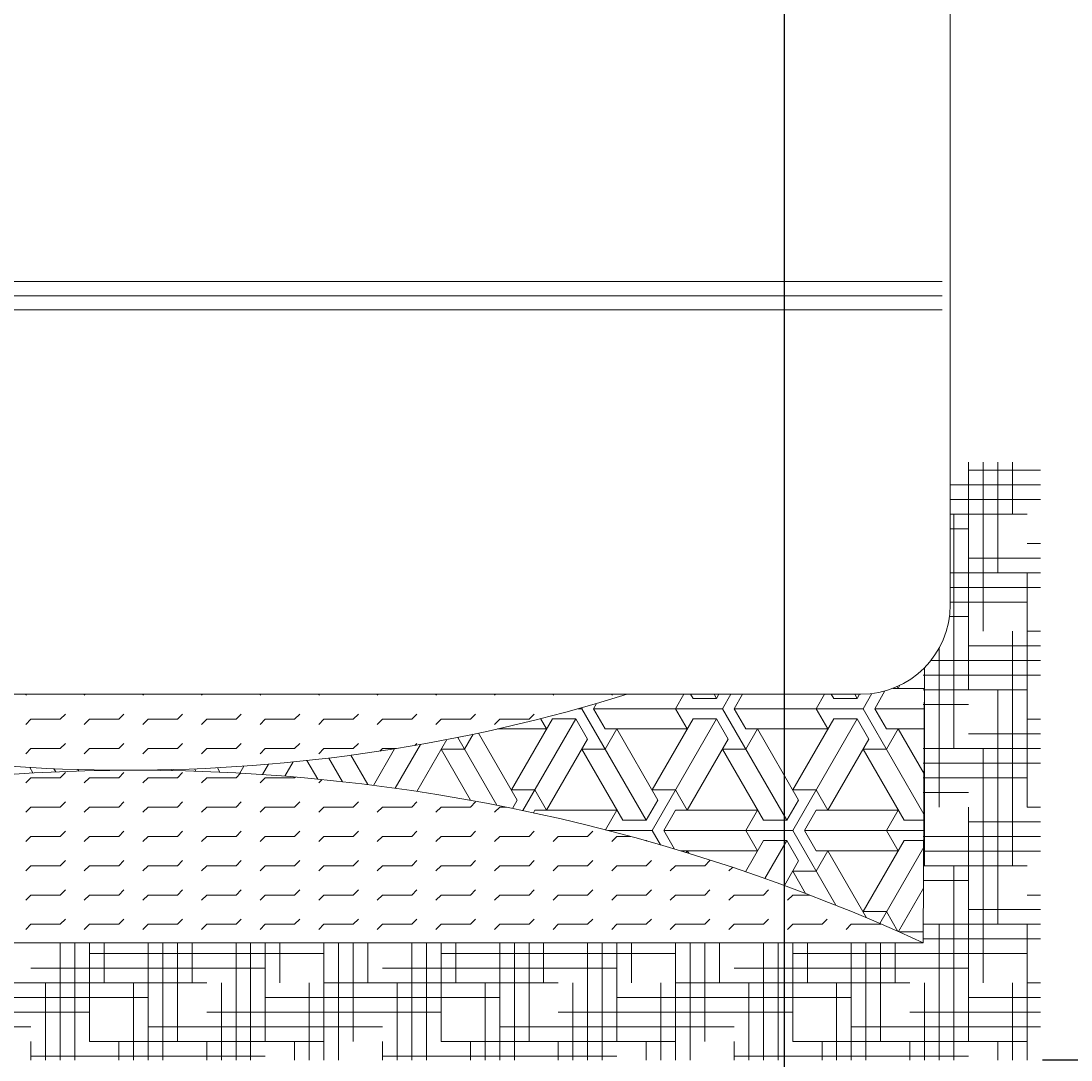
# Model space of a CAD drawing. Units: inches. Extents: x -1517 to -668, y -425 to 52.
# Tile 9 of 13: x -1161 to -1129, y -63 to -32. Entities that reach past the tile are written whole.
import ezdxf

# ---------------------------------------------------------------- set-up
doc = ezdxf.new("R2010")
doc.units = ezdxf.units.IN
doc.header["$MEASUREMENT"] = 0
doc.layers.add('A-ANNO-DIMS', color=2, linetype='Continuous', lineweight=18)
doc.layers.add('furniture block', color=8, linetype='Continuous', lineweight=18)
doc.styles.get("Standard").update_dxf_attribs({"font": 'arial.ttf'})
doc.dimstyles.get("Standard").update_dxf_attribs({"dimtxt": 0.18, "dimasz": 0.18, "dimexe": 0.18, "dimexo": 0.0625, "dimgap": 0.09, "dimtad": 0, "dimtih": 1, "dimtoh": 1, "dimdec": 4, "dimzin": 0, "dimdsep": 46, "dimlunit": 4, "dimtxsty": 'Standard', "dimcen": 0.09, "dimadec": 0, "dimazin": 0, "dimtfac": 1, "dimtdec": 4, "dimtofl": 0, "dimtmove": 0, "dimatfit": 3, "dimfxl": 1, "dimtolj": 1, "dimtzin": 0, "dimarcsym": 0})

# ---------------------------------------------------------------- blocks, each defined once
blk = doc.blocks.new('A$C62731D1C')
for p, q in [((1.46787, 2.14084, 0.68571), (1.46787, 0.38824, 0.68571)), ((0.10613, 0.66415, 0.68571), (1.46095, 0.66415, 0.68571)), ((0.10613, 0.65215, 0.68571), (1.46095, 0.65215, 0.68571)), ((0.10613, 0.64015, 0.68571), (1.46095, 0.64015, 0.68571)), ((1.4835, 0.31577, 0.68571), (1.4835, 0.50998, 0.68571)), ((1.4835, 0.50327, 0.68571), (1.54488, 0.50327, 0.68571)), ((1.496, 0.36577, 0.68571), (1.496, 0.50998, 0.68571)), ((1.5085, 0.41577, 0.68571), (1.5085, 0.50998, 0.68571)), ((1.521, 0.46577, 0.68571), (1.521, 0.50998, 0.68571)), ((1.46787, 0.49077, 0.68571), (1.54488, 0.49077, 0.68571)), ((1.46787, 0.47827, 0.68571), (1.54488, 0.47827, 0.68571)), ((1.46787, 0.46577, 0.68571), (1.5335, 0.46577, 0.68571)), ((1.471, 0.26577, 0.68571), (1.471, 0.46577, 0.68571)), ((1.46787, 0.45327, 0.68571), (1.4835, 0.45327, 0.68571)), ((1.5335, 0.44077, 0.68571), (1.54488, 0.44077, 0.68571)), ((1.4835, 0.42827, 0.68571), (1.54488, 0.42827, 0.68571)), ((1.46787, 0.41577, 0.68571), (1.54488, 0.41577, 0.68571)), ((1.5335, 0.21577, 0.68571), (1.5335, 0.41577, 0.68571)), ((1.46787, 0.40327, 0.68571), (1.54488, 0.40327, 0.68571)), ((1.46787, 0.39077, 0.68571), (1.5335, 0.39077, 0.68571)), ((1.46722, 0.37827, 0.68571), (1.4835, 0.37827, 0.68571)), ((1.521, 0.16577, 0.68571), (1.521, 0.36577, 0.68571)), ((1.5335, 0.36577, 0.68571), (1.54488, 0.36577, 0.68571)), ((1.4585, 0.21577, 0.68571), (1.4585, 0.35163, 0.68571)), ((1.4835, 0.35327, 0.68571), (1.54488, 0.35327, 0.68571)), ((1.45128, 0.34077, 0.68571), (1.54488, 0.34077, 0.68571)), ((1.446, 0.33481, 0.68571), (1.44488, 0.1, 0.68571)), ((1.446, 0.16577, 0.68571), (1.446, 0.33481, 0.68571)), ((1.44488, 0.32827, 0.68571), (1.54488, 0.32827, 0.68571)), ((1.4035, 0.29977, 0.68571), (1.41221, 0.31486, 0.68571)), ((1.41896, 0.31709, 0.68571), (1.44592, 0.31709, 0.68571)), ((1.42263, 0.31861, 0.68571), (1.4235, 0.31709, 0.68571)), ((1.42502, 0.31973, 0.68571), (1.4235, 0.31709, 0.68571)), ((1.44488, 0.31577, 0.68571), (1.5335, 0.31577, 0.68571)), ((1.5085, 0.11577, 0.68571), (1.5085, 0.31577, 0.68571)), ((1.39167, 0.31204, 0.68571), (0.17247, 0.31204, 0.68571)), ((0.67908, 0.31135, 0.68571), (0.67977, 0.31204, 0.68571)), ((0.72908, 0.31135, 0.68571), (0.72977, 0.31204, 0.68571)), ((0.77908, 0.31135, 0.68571), (0.77977, 0.31204, 0.68571)), ((0.82908, 0.31135, 0.68571), (0.82977, 0.31204, 0.68571)), ((0.87908, 0.31135, 0.68571), (0.87977, 0.31204, 0.68571)), ((0.92908, 0.31135, 0.68571), (0.92977, 0.31204, 0.68571)), ((0.97908, 0.31135, 0.68571), (0.97977, 0.31204, 0.68571)), ((1.02908, 0.31135, 0.68571), (1.02977, 0.31204, 0.68571)), ((1.07908, 0.31135, 0.68571), (1.07977, 0.31204, 0.68571)), ((1.12908, 0.31135, 0.68571), (1.12977, 0.31204, 0.68571)), ((1.17908, 0.31135, 0.68571), (1.17977, 0.31204, 0.68571)), ((1.2335, 0.29977, 0.68571), (1.24058, 0.31204, 0.68571)), ((1.2485, 0.30843, 0.68571), (1.24642, 0.31204, 0.68571)), ((1.2685, 0.30843, 0.68571), (1.2485, 0.30843, 0.68571)), ((1.26642, 0.31204, 0.68571), (1.2685, 0.30843, 0.68571)), ((1.2685, 0.30843, 0.68571), (1.27058, 0.31204, 0.68571)), ((1.2735, 0.29977, 0.68571), (1.28058, 0.31204, 0.68571)), ((1.2835, 0.29977, 0.68571), (1.29058, 0.31204, 0.68571)), ((1.3535, 0.29977, 0.68571), (1.36058, 0.31204, 0.68571)), ((1.3685, 0.30843, 0.68571), (1.36642, 0.31204, 0.68571)), ((1.3885, 0.30843, 0.68571), (1.3685, 0.30843, 0.68571)), ((1.38642, 0.31204, 0.68571), (1.3885, 0.30843, 0.68571)), ((1.3885, 0.30843, 0.68571), (1.39058, 0.31204, 0.68571)), ((1.3935, 0.29977, 0.68571), (1.40091, 0.3126, 0.68571)), ((1.1535, 0.29977, 0.68571), (1.15051, 0.29977, 0.68571)), ((1.1535, 0.29977, 0.68571), (1.15408, 0.30077, 0.68571)), ((1.1535, 0.29977, 0.68571), (1.2085, 0.20451, 0.68571)), ((1.1635, 0.29977, 0.68571), (1.16604, 0.30418, 0.68571)), ((1.2735, 0.29977, 0.68571), (1.1635, 0.29977, 0.68571)), ((1.1635, 0.29977, 0.68571), (1.1735, 0.28245, 0.68571)), ((1.2335, 0.29977, 0.68571), (1.2435, 0.28245, 0.68571)), ((1.2735, 0.29977, 0.68571), (1.3285, 0.20451, 0.68571)), ((1.3935, 0.29977, 0.68571), (1.2835, 0.29977, 0.68571)), ((1.2835, 0.29977, 0.68571), (1.2935, 0.28245, 0.68571)), ((1.3535, 0.29977, 0.68571), (1.3635, 0.28245, 0.68571)), ((1.3935, 0.29977, 0.68571), (1.44541, 0.20987, 0.68571)), ((1.44583, 0.29977, 0.68571), (1.4035, 0.29977, 0.68571)), ((1.4035, 0.29977, 0.68571), (1.4135, 0.28245, 0.68571)), ((1.44488, 0.30327, 0.68571), (1.4835, 0.30327, 0.68571)), ((0.67908, 0.28635, 0.68571), (0.6835, 0.29077, 0.68571)), ((0.6835, 0.29077, 0.68571), (0.7085, 0.29077, 0.68571)), ((0.7085, 0.29077, 0.68571), (0.71292, 0.29519, 0.68571)), ((0.72908, 0.28635, 0.68571), (0.7335, 0.29077, 0.68571)), ((0.7335, 0.29077, 0.68571), (0.7585, 0.29077, 0.68571)), ((0.7585, 0.29077, 0.68571), (0.76292, 0.29519, 0.68571)), ((0.77908, 0.28635, 0.68571), (0.7835, 0.29077, 0.68571)), ((0.7835, 0.29077, 0.68571), (0.8085, 0.29077, 0.68571)), ((0.8085, 0.29077, 0.68571), (0.81292, 0.29519, 0.68571)), ((0.82908, 0.28635, 0.68571), (0.8335, 0.29077, 0.68571)), ((0.8335, 0.29077, 0.68571), (0.8585, 0.29077, 0.68571)), ((0.8585, 0.29077, 0.68571), (0.86292, 0.29519, 0.68571)), ((0.87908, 0.28635, 0.68571), (0.8835, 0.29077, 0.68571)), ((0.8835, 0.29077, 0.68571), (0.9085, 0.29077, 0.68571)), ((0.9085, 0.29077, 0.68571), (0.91292, 0.29519, 0.68571)), ((0.92908, 0.28635, 0.68571), (0.9335, 0.29077, 0.68571)), ((0.9335, 0.29077, 0.68571), (0.9585, 0.29077, 0.68571)), ((0.9585, 0.29077, 0.68571), (0.96292, 0.29519, 0.68571)), ((0.97908, 0.28635, 0.68571), (0.9835, 0.29077, 0.68571)), ((0.9835, 0.29077, 0.68571), (1.0085, 0.29077, 0.68571)), ((1.0085, 0.29077, 0.68571), (1.01292, 0.29519, 0.68571)), ((1.02908, 0.28635, 0.68571), (1.0335, 0.29077, 0.68571)), ((1.0335, 0.29077, 0.68571), (1.0585, 0.29077, 0.68571)), ((1.0585, 0.29077, 0.68571), (1.06292, 0.29519, 0.68571)), ((1.07908, 0.28635, 0.68571), (1.0835, 0.29077, 0.68571)), ((1.0835, 0.29077, 0.68571), (1.1085, 0.29077, 0.68571)), ((1.1285, 0.29111, 0.68571), (1.0935, 0.23049, 0.68571)), ((1.10332, 0.21286, 0.68571), (1.1485, 0.29111, 0.68571)), ((1.1085, 0.29077, 0.68571), (1.11292, 0.29519, 0.68571)), ((1.11842, 0.29126, 0.68571), (1.1235, 0.28245, 0.68571)), ((1.1485, 0.29111, 0.68571), (1.1285, 0.29111, 0.68571)), ((1.1485, 0.29111, 0.68571), (1.1585, 0.27379, 0.68571)), ((1.2135, 0.19585, 0.68571), (1.2685, 0.29111, 0.68571)), ((1.2485, 0.29111, 0.68571), (1.2135, 0.23049, 0.68571)), ((1.2685, 0.29111, 0.68571), (1.2485, 0.29111, 0.68571)), ((1.2685, 0.29111, 0.68571), (1.2785, 0.27379, 0.68571)), ((1.3335, 0.19585, 0.68571), (1.3885, 0.29111, 0.68571)), ((1.3685, 0.29111, 0.68571), (1.3335, 0.23049, 0.68571)), ((1.3885, 0.29111, 0.68571), (1.3685, 0.29111, 0.68571)), ((1.3885, 0.29111, 0.68571), (1.3985, 0.27379, 0.68571)), ((1.5335, 0.29077, 0.68571), (1.54488, 0.29077, 0.68571)), ((1.0535, 0.26513, 0.68571), (1.06091, 0.27796, 0.68571)), ((1.0985, 0.22183, 0.68571), (1.06553, 0.27894, 0.68571)), ((1.08156, 0.28245, 0.68571), (1.1235, 0.28245, 0.68571)), ((1.1735, 0.26513, 0.68571), (1.1835, 0.28245, 0.68571)), ((1.1735, 0.28245, 0.68571), (1.2435, 0.28245, 0.68571)), ((1.2185, 0.22183, 0.68571), (1.1835, 0.28245, 0.68571)), ((1.2935, 0.26513, 0.68571), (1.3035, 0.28245, 0.68571)), ((1.2935, 0.28245, 0.68571), (1.3635, 0.28245, 0.68571)), ((1.3385, 0.22183, 0.68571), (1.3035, 0.28245, 0.68571)), ((1.4135, 0.26513, 0.68571), (1.4235, 0.28245, 0.68571)), ((1.4135, 0.28245, 0.68571), (1.44575, 0.28245, 0.68571)), ((1.44557, 0.24423, 0.68571), (1.4235, 0.28245, 0.68571)), ((1.4835, 0.27827, 0.68571), (1.54488, 0.27827, 0.68571)), ((0.7085, 0.26577, 0.68571), (0.71292, 0.27019, 0.68571)), ((0.7585, 0.26577, 0.68571), (0.76292, 0.27019, 0.68571)), ((0.8085, 0.26577, 0.68571), (0.81292, 0.27019, 0.68571)), ((0.8585, 0.26577, 0.68571), (0.86292, 0.27019, 0.68571)), ((0.9085, 0.26577, 0.68571), (0.91292, 0.27019, 0.68571)), ((0.9585, 0.26577, 0.68571), (0.96292, 0.27019, 0.68571)), ((0.9943, 0.23188, 0.68571), (1.01588, 0.26926, 0.68571)), ((1.01117, 0.26843, 0.68571), (1.01292, 0.27019, 0.68571)), ((1.03828, 0.2734, 0.68571), (1.01275, 0.2292, 0.68571)), ((1.04766, 0.27525, 0.68571), (1.08108, 0.21737, 0.68571)), ((1.1585, 0.27379, 0.68571), (1.1235, 0.21317, 0.68571)), ((1.2785, 0.27379, 0.68571), (1.2435, 0.21317, 0.68571)), ((1.3985, 0.27379, 0.68571), (1.3635, 0.21317, 0.68571)), ((0.67908, 0.26135, 0.68571), (0.6835, 0.26577, 0.68571)), ((0.6835, 0.26577, 0.68571), (0.7085, 0.26577, 0.68571)), ((0.72908, 0.26135, 0.68571), (0.7335, 0.26577, 0.68571)), ((0.7335, 0.26577, 0.68571), (0.7585, 0.26577, 0.68571)), ((0.77908, 0.26135, 0.68571), (0.7835, 0.26577, 0.68571)), ((0.7835, 0.26577, 0.68571), (0.8085, 0.26577, 0.68571)), ((0.82908, 0.26135, 0.68571), (0.8335, 0.26577, 0.68571)), ((0.8335, 0.26577, 0.68571), (0.8585, 0.26577, 0.68571)), ((0.87908, 0.26135, 0.68571), (0.8835, 0.26577, 0.68571)), ((0.8835, 0.26577, 0.68571), (0.9085, 0.26577, 0.68571)), ((0.92908, 0.26135, 0.68571), (0.9335, 0.26577, 0.68571)), ((0.9335, 0.26577, 0.68571), (0.9585, 0.26577, 0.68571)), ((0.97092, 0.23496, 0.68571), (0.95645, 0.26002, 0.68571)), ((0.99372, 0.26552, 0.68571), (0.97573, 0.23435, 0.68571)), ((0.98131, 0.26358, 0.68571), (0.9835, 0.26577, 0.68571)), ((0.9835, 0.26577, 0.68571), (0.99527, 0.26577, 0.68571)), ((1.0535, 0.26513, 0.68571), (1.0335, 0.26513, 0.68571)), ((1.05864, 0.22159, 0.68571), (1.0335, 0.26513, 0.68571)), ((1.1735, 0.26513, 0.68571), (1.1535, 0.26513, 0.68571)), ((1.1885, 0.20451, 0.68571), (1.1535, 0.26513, 0.68571)), ((1.2935, 0.26513, 0.68571), (1.2735, 0.26513, 0.68571)), ((1.3085, 0.20451, 0.68571), (1.2735, 0.26513, 0.68571)), ((1.4135, 0.26513, 0.68571), (1.3935, 0.26513, 0.68571)), ((1.4285, 0.20451, 0.68571), (1.3935, 0.26513, 0.68571)), ((1.44488, 0.26577, 0.68571), (1.54488, 0.26577, 0.68571)), ((1.496, 0.06577, 0.68571), (1.496, 0.26577, 0.68571)), ((0.88105, 0.24357, 0.68571), (0.88611, 0.25234, 0.68571)), ((0.90723, 0.25428, 0.68571), (0.90024, 0.24216, 0.68571)), ((0.92819, 0.23969, 0.68571), (0.91906, 0.2555, 0.68571)), ((0.93782, 0.25765, 0.68571), (0.94947, 0.23748, 0.68571)), ((1.44488, 0.25327, 0.68571), (1.54488, 0.25327, 0.68571)), ((0.6852, 0.24488, 0.68571), (0.6825, 0.24954, 0.68571)), ((0.70309, 0.24852, 0.68571), (0.70465, 0.24582, 0.68571)), ((0.7085, 0.24077, 0.68571), (0.71292, 0.24519, 0.68571)), ((0.72425, 0.24652, 0.68571), (0.72351, 0.24779, 0.68571)), ((0.74324, 0.24737, 0.68571), (0.74302, 0.24697, 0.68571)), ((0.7585, 0.24077, 0.68571), (0.76292, 0.24519, 0.68571)), ((0.78322, 0.24733, 0.68571), (0.78315, 0.24721, 0.68571)), ((0.80401, 0.24693, 0.68571), (0.80355, 0.24773, 0.68571)), ((0.8085, 0.24077, 0.68571), (0.81292, 0.24519, 0.68571)), ((0.82316, 0.2484, 0.68571), (0.82431, 0.24641, 0.68571)), ((0.84477, 0.24562, 0.68571), (0.84263, 0.24932, 0.68571)), ((0.8585, 0.24077, 0.68571), (0.86246, 0.24472, 0.68571)), ((0.86518, 0.25072, 0.68571), (0.86174, 0.24476, 0.68571)), ((0.67908, 0.23635, 0.68571), (0.6835, 0.24077, 0.68571)), ((0.6835, 0.24077, 0.68571), (0.7085, 0.24077, 0.68571)), ((0.72908, 0.23635, 0.68571), (0.7335, 0.24077, 0.68571)), ((0.7335, 0.24077, 0.68571), (0.7585, 0.24077, 0.68571)), ((0.77908, 0.23635, 0.68571), (0.7835, 0.24077, 0.68571)), ((0.7835, 0.24077, 0.68571), (0.8085, 0.24077, 0.68571)), ((0.82908, 0.23635, 0.68571), (0.8335, 0.24077, 0.68571)), ((0.8335, 0.24077, 0.68571), (0.8585, 0.24077, 0.68571)), ((0.87908, 0.23635, 0.68571), (0.8835, 0.24077, 0.68571)), ((0.8835, 0.24077, 0.68571), (0.9085, 0.24077, 0.68571)), ((0.9085, 0.24077, 0.68571), (0.90916, 0.24143, 0.68571)), ((0.92908, 0.23635, 0.68571), (0.93204, 0.23931, 0.68571)), ((1.44488, 0.24077, 0.68571), (1.5335, 0.24077, 0.68571)), ((1.1135, 0.23049, 0.68571), (1.0935, 0.23049, 0.68571)), ((1.1135, 0.23049, 0.68571), (1.1235, 0.21317, 0.68571)), ((1.2335, 0.23049, 0.68571), (1.2135, 0.23049, 0.68571)), ((1.2335, 0.23049, 0.68571), (1.2435, 0.21317, 0.68571)), ((1.3535, 0.23049, 0.68571), (1.3335, 0.23049, 0.68571)), ((1.3535, 0.23049, 0.68571), (1.3635, 0.21317, 0.68571)), ((1.44488, 0.22827, 0.68571), (1.4835, 0.22827, 0.68571)), ((0.67908, 0.21135, 0.68571), (0.6835, 0.21577, 0.68571)), ((0.6835, 0.21577, 0.68571), (0.7085, 0.21577, 0.68571)), ((0.7085, 0.21577, 0.68571), (0.71292, 0.22019, 0.68571)), ((0.72908, 0.21135, 0.68571), (0.7335, 0.21577, 0.68571)), ((0.7335, 0.21577, 0.68571), (0.7585, 0.21577, 0.68571)), ((0.7585, 0.21577, 0.68571), (0.76292, 0.22019, 0.68571)), ((0.77908, 0.21135, 0.68571), (0.7835, 0.21577, 0.68571)), ((0.7835, 0.21577, 0.68571), (0.8085, 0.21577, 0.68571)), ((0.8085, 0.21577, 0.68571), (0.81292, 0.22019, 0.68571)), ((0.82908, 0.21135, 0.68571), (0.8335, 0.21577, 0.68571)), ((0.8335, 0.21577, 0.68571), (0.8585, 0.21577, 0.68571)), ((0.8585, 0.21577, 0.68571), (0.86292, 0.22019, 0.68571)), ((0.87908, 0.21135, 0.68571), (0.8835, 0.21577, 0.68571)), ((0.8835, 0.21577, 0.68571), (0.9085, 0.21577, 0.68571)), ((0.9085, 0.21577, 0.68571), (0.91292, 0.22019, 0.68571)), ((0.92908, 0.21135, 0.68571), (0.9335, 0.21577, 0.68571)), ((0.9335, 0.21577, 0.68571), (0.9585, 0.21577, 0.68571)), ((0.9585, 0.21577, 0.68571), (0.96292, 0.22019, 0.68571)), ((0.97908, 0.21135, 0.68571), (0.9835, 0.21577, 0.68571)), ((0.9835, 0.21577, 0.68571), (1.0085, 0.21577, 0.68571)), ((1.0085, 0.21577, 0.68571), (1.01292, 0.22019, 0.68571)), ((1.02908, 0.21135, 0.68571), (1.0335, 0.21577, 0.68571)), ((1.0335, 0.21577, 0.68571), (1.0585, 0.21577, 0.68571)), ((1.0585, 0.21577, 0.68571), (1.06292, 0.22019, 0.68571)), ((1.07908, 0.21135, 0.68571), (1.0835, 0.21577, 0.68571)), ((1.0835, 0.21577, 0.68571), (1.08915, 0.21577, 0.68571)), ((1.09439, 0.21471, 0.68571), (1.0985, 0.22183, 0.68571)), ((1.2085, 0.20451, 0.68571), (1.2185, 0.22183, 0.68571)), ((1.3285, 0.20451, 0.68571), (1.3385, 0.22183, 0.68571)), ((1.4835, 0.01577, 0.68571), (1.4835, 0.21577, 0.68571)), ((1.5335, 0.21577, 0.68571), (1.54488, 0.21577, 0.68571)), ((1.11222, 0.21096, 0.68571), (1.1135, 0.21317, 0.68571)), ((1.1135, 0.21317, 0.68571), (1.1835, 0.21317, 0.68571)), ((1.17381, 0.19638, 0.68571), (1.1835, 0.21317, 0.68571)), ((1.2235, 0.19585, 0.68571), (1.2335, 0.21317, 0.68571)), ((1.2335, 0.21317, 0.68571), (1.3035, 0.21317, 0.68571)), ((1.2935, 0.19585, 0.68571), (1.3035, 0.21317, 0.68571)), ((1.3435, 0.19585, 0.68571), (1.3535, 0.21317, 0.68571)), ((1.3535, 0.21317, 0.68571), (1.4235, 0.21317, 0.68571)), ((1.4135, 0.19585, 0.68571), (1.4235, 0.21317, 0.68571)), ((1.2085, 0.20451, 0.68571), (1.1885, 0.20451, 0.68571)), ((1.3285, 0.20451, 0.68571), (1.3085, 0.20451, 0.68571)), ((1.44538, 0.20451, 0.68571), (1.4285, 0.20451, 0.68571)), ((1.4835, 0.20327, 0.68571), (1.54488, 0.20327, 0.68571)), ((0.67908, 0.18635, 0.68571), (0.6835, 0.19077, 0.68571)), ((0.6835, 0.19077, 0.68571), (0.7085, 0.19077, 0.68571)), ((0.7085, 0.19077, 0.68571), (0.71292, 0.19519, 0.68571)), ((0.72908, 0.18635, 0.68571), (0.7335, 0.19077, 0.68571)), ((0.7335, 0.19077, 0.68571), (0.7585, 0.19077, 0.68571)), ((0.7585, 0.19077, 0.68571), (0.76292, 0.19519, 0.68571)), ((0.77908, 0.18635, 0.68571), (0.7835, 0.19077, 0.68571)), ((0.7835, 0.19077, 0.68571), (0.8085, 0.19077, 0.68571)), ((0.8085, 0.19077, 0.68571), (0.81292, 0.19519, 0.68571)), ((0.82908, 0.18635, 0.68571), (0.8335, 0.19077, 0.68571)), ((0.8335, 0.19077, 0.68571), (0.8585, 0.19077, 0.68571)), ((0.8585, 0.19077, 0.68571), (0.86292, 0.19519, 0.68571)), ((0.87908, 0.18635, 0.68571), (0.8835, 0.19077, 0.68571)), ((0.8835, 0.19077, 0.68571), (0.9085, 0.19077, 0.68571)), ((0.9085, 0.19077, 0.68571), (0.91292, 0.19519, 0.68571)), ((0.92908, 0.18635, 0.68571), (0.9335, 0.19077, 0.68571)), ((0.9335, 0.19077, 0.68571), (0.9585, 0.19077, 0.68571)), ((0.9585, 0.19077, 0.68571), (0.96292, 0.19519, 0.68571)), ((0.97908, 0.18635, 0.68571), (0.9835, 0.19077, 0.68571)), ((0.9835, 0.19077, 0.68571), (1.0085, 0.19077, 0.68571)), ((1.0085, 0.19077, 0.68571), (1.01292, 0.19519, 0.68571)), ((1.02908, 0.18635, 0.68571), (1.0335, 0.19077, 0.68571)), ((1.0335, 0.19077, 0.68571), (1.0585, 0.19077, 0.68571)), ((1.0585, 0.19077, 0.68571), (1.06292, 0.19519, 0.68571)), ((1.07908, 0.18635, 0.68571), (1.0835, 0.19077, 0.68571)), ((1.0835, 0.19077, 0.68571), (1.1085, 0.19077, 0.68571)), ((1.1085, 0.19077, 0.68571), (1.11292, 0.19519, 0.68571)), ((1.12908, 0.18635, 0.68571), (1.1335, 0.19077, 0.68571)), ((1.1335, 0.19077, 0.68571), (1.1585, 0.19077, 0.68571)), ((1.1585, 0.19077, 0.68571), (1.16292, 0.19519, 0.68571)), ((1.2135, 0.19585, 0.68571), (1.17586, 0.19585, 0.68571)), ((1.17908, 0.18635, 0.68571), (1.1835, 0.19077, 0.68571)), ((1.1835, 0.19077, 0.68571), (1.195, 0.19077, 0.68571)), ((1.2135, 0.19585, 0.68571), (1.22059, 0.18358, 0.68571)), ((1.3335, 0.19585, 0.68571), (1.2235, 0.19585, 0.68571)), ((1.2235, 0.19585, 0.68571), (1.23263, 0.18003, 0.68571)), ((1.2935, 0.19585, 0.68571), (1.3035, 0.17853, 0.68571)), ((1.3335, 0.19585, 0.68571), (1.37035, 0.13204, 0.68571)), ((1.44534, 0.19585, 0.68571), (1.3435, 0.19585, 0.68571)), ((1.3435, 0.19585, 0.68571), (1.3535, 0.17853, 0.68571)), ((1.4135, 0.19585, 0.68571), (1.4235, 0.17853, 0.68571)), ((1.44488, 0.19077, 0.68571), (1.54488, 0.19077, 0.68571)), ((1.2085, 0.18719, 0.68571), (1.20794, 0.18719, 0.68571)), ((1.20842, 0.18705, 0.68571), (1.2085, 0.18719, 0.68571)), ((1.2085, 0.18719, 0.68571), (1.20861, 0.187, 0.68571)), ((1.3085, 0.18719, 0.68571), (1.29318, 0.16065, 0.68571)), ((1.3285, 0.18719, 0.68571), (1.3085, 0.18719, 0.68571)), ((1.30983, 0.15486, 0.68571), (1.3285, 0.18719, 0.68571)), ((1.3285, 0.18719, 0.68571), (1.3385, 0.16987, 0.68571)), ((1.4285, 0.18719, 0.68571), (1.3935, 0.12657, 0.68571)), ((1.40771, 0.11653, 0.68571), (1.44527, 0.1816, 0.68571)), ((1.4453, 0.18719, 0.68571), (1.4285, 0.18719, 0.68571)), ((1.23764, 0.17853, 0.68571), (1.3035, 0.17853, 0.68571)), ((1.24263, 0.17702, 0.68571), (1.2435, 0.17853, 0.68571)), ((1.24475, 0.17637, 0.68571), (1.2435, 0.17853, 0.68571)), ((1.3535, 0.16121, 0.68571), (1.3635, 0.17853, 0.68571)), ((1.3535, 0.17853, 0.68571), (1.4235, 0.17853, 0.68571)), ((1.39656, 0.12128, 0.68571), (1.3635, 0.17853, 0.68571)), ((1.44488, 0.17827, 0.68571), (1.54488, 0.17827, 0.68571)), ((0.67908, 0.16135, 0.68571), (0.6835, 0.16577, 0.68571)), ((0.6835, 0.16577, 0.68571), (0.7085, 0.16577, 0.68571)), ((0.7085, 0.16577, 0.68571), (0.71292, 0.17019, 0.68571)), ((0.72908, 0.16135, 0.68571), (0.7335, 0.16577, 0.68571)), ((0.7335, 0.16577, 0.68571), (0.7585, 0.16577, 0.68571)), ((0.7585, 0.16577, 0.68571), (0.76292, 0.17019, 0.68571)), ((0.77908, 0.16135, 0.68571), (0.7835, 0.16577, 0.68571)), ((0.7835, 0.16577, 0.68571), (0.8085, 0.16577, 0.68571)), ((0.8085, 0.16577, 0.68571), (0.81292, 0.17019, 0.68571)), ((0.82908, 0.16135, 0.68571), (0.8335, 0.16577, 0.68571)), ((0.8335, 0.16577, 0.68571), (0.8585, 0.16577, 0.68571)), ((0.8585, 0.16577, 0.68571), (0.86292, 0.17019, 0.68571)), ((0.87908, 0.16135, 0.68571), (0.8835, 0.16577, 0.68571)), ((0.8835, 0.16577, 0.68571), (0.9085, 0.16577, 0.68571)), ((0.9085, 0.16577, 0.68571), (0.91292, 0.17019, 0.68571)), ((0.92908, 0.16135, 0.68571), (0.9335, 0.16577, 0.68571)), ((0.9335, 0.16577, 0.68571), (0.9585, 0.16577, 0.68571)), ((0.9585, 0.16577, 0.68571), (0.96292, 0.17019, 0.68571)), ((0.97908, 0.16135, 0.68571), (0.9835, 0.16577, 0.68571)), ((0.9835, 0.16577, 0.68571), (1.0085, 0.16577, 0.68571)), ((1.0085, 0.16577, 0.68571), (1.01292, 0.17019, 0.68571)), ((1.02908, 0.16135, 0.68571), (1.0335, 0.16577, 0.68571)), ((1.0335, 0.16577, 0.68571), (1.0585, 0.16577, 0.68571)), ((1.0585, 0.16577, 0.68571), (1.06292, 0.17019, 0.68571)), ((1.07908, 0.16135, 0.68571), (1.0835, 0.16577, 0.68571)), ((1.0835, 0.16577, 0.68571), (1.1085, 0.16577, 0.68571)), ((1.1085, 0.16577, 0.68571), (1.11292, 0.17019, 0.68571)), ((1.12908, 0.16135, 0.68571), (1.1335, 0.16577, 0.68571)), ((1.1335, 0.16577, 0.68571), (1.1585, 0.16577, 0.68571)), ((1.1585, 0.16577, 0.68571), (1.16292, 0.17019, 0.68571)), ((1.17908, 0.16135, 0.68571), (1.1835, 0.16577, 0.68571)), ((1.1835, 0.16577, 0.68571), (1.2085, 0.16577, 0.68571)), ((1.2085, 0.16577, 0.68571), (1.21292, 0.17019, 0.68571)), ((1.22908, 0.16135, 0.68571), (1.2335, 0.16577, 0.68571)), ((1.2335, 0.16577, 0.68571), (1.2585, 0.16577, 0.68571)), ((1.2585, 0.16577, 0.68571), (1.26292, 0.17019, 0.68571)), ((1.27908, 0.16135, 0.68571), (1.28212, 0.16439, 0.68571)), ((1.3385, 0.16987, 0.68571), (1.32639, 0.14889, 0.68571)), ((1.44488, 0.16577, 0.68571), (1.5335, 0.16577, 0.68571)), ((1.471, 0, 0.68571), (1.471, 0.16577, 0.68571)), ((1.3535, 0.16121, 0.68571), (1.3335, 0.16121, 0.68571)), ((1.34453, 0.14211, 0.68571), (1.3335, 0.16121, 0.68571)), ((1.44488, 0.15327, 0.68571), (1.4835, 0.15327, 0.68571)), ((0.7085, 0.14077, 0.68571), (0.71292, 0.14519, 0.68571)), ((0.7585, 0.14077, 0.68571), (0.76292, 0.14519, 0.68571)), ((0.8085, 0.14077, 0.68571), (0.81292, 0.14519, 0.68571)), ((0.8585, 0.14077, 0.68571), (0.86292, 0.14519, 0.68571)), ((0.9085, 0.14077, 0.68571), (0.91292, 0.14519, 0.68571)), ((0.9585, 0.14077, 0.68571), (0.96292, 0.14519, 0.68571)), ((1.0085, 0.14077, 0.68571), (1.01292, 0.14519, 0.68571)), ((1.0585, 0.14077, 0.68571), (1.06292, 0.14519, 0.68571)), ((1.1085, 0.14077, 0.68571), (1.11292, 0.14519, 0.68571)), ((1.1585, 0.14077, 0.68571), (1.16292, 0.14519, 0.68571)), ((1.2085, 0.14077, 0.68571), (1.21292, 0.14519, 0.68571)), ((1.2585, 0.14077, 0.68571), (1.26292, 0.14519, 0.68571)), ((1.3085, 0.14077, 0.68571), (1.31292, 0.14519, 0.68571)), ((1.44511, 0.14667, 0.68571), (1.42369, 0.10957, 0.68571)), ((0.67908, 0.13635, 0.68571), (0.6835, 0.14077, 0.68571)), ((0.6835, 0.14077, 0.68571), (0.7085, 0.14077, 0.68571)), ((0.72908, 0.13635, 0.68571), (0.7335, 0.14077, 0.68571)), ((0.7335, 0.14077, 0.68571), (0.7585, 0.14077, 0.68571)), ((0.77908, 0.13635, 0.68571), (0.7835, 0.14077, 0.68571)), ((0.7835, 0.14077, 0.68571), (0.8085, 0.14077, 0.68571)), ((0.82908, 0.13635, 0.68571), (0.8335, 0.14077, 0.68571)), ((0.8335, 0.14077, 0.68571), (0.8585, 0.14077, 0.68571)), ((0.87908, 0.13635, 0.68571), (0.8835, 0.14077, 0.68571)), ((0.8835, 0.14077, 0.68571), (0.9085, 0.14077, 0.68571)), ((0.92908, 0.13635, 0.68571), (0.9335, 0.14077, 0.68571)), ((0.9335, 0.14077, 0.68571), (0.9585, 0.14077, 0.68571)), ((0.97908, 0.13635, 0.68571), (0.9835, 0.14077, 0.68571)), ((0.9835, 0.14077, 0.68571), (1.0085, 0.14077, 0.68571)), ((1.02908, 0.13635, 0.68571), (1.0335, 0.14077, 0.68571)), ((1.0335, 0.14077, 0.68571), (1.0585, 0.14077, 0.68571)), ((1.07908, 0.13635, 0.68571), (1.0835, 0.14077, 0.68571)), ((1.0835, 0.14077, 0.68571), (1.1085, 0.14077, 0.68571)), ((1.12908, 0.13635, 0.68571), (1.1335, 0.14077, 0.68571)), ((1.1335, 0.14077, 0.68571), (1.1585, 0.14077, 0.68571)), ((1.17908, 0.13635, 0.68571), (1.1835, 0.14077, 0.68571)), ((1.1835, 0.14077, 0.68571), (1.2085, 0.14077, 0.68571)), ((1.22908, 0.13635, 0.68571), (1.2335, 0.14077, 0.68571)), ((1.2335, 0.14077, 0.68571), (1.2585, 0.14077, 0.68571)), ((1.27908, 0.13635, 0.68571), (1.2835, 0.14077, 0.68571)), ((1.2835, 0.14077, 0.68571), (1.3085, 0.14077, 0.68571)), ((1.32908, 0.13635, 0.68571), (1.3335, 0.14077, 0.68571)), ((1.3335, 0.14077, 0.68571), (1.34805, 0.14077, 0.68571)), ((1.5335, 0.14077, 0.68571), (1.54488, 0.14077, 0.68571)), ((1.4135, 0.12657, 0.68571), (1.3935, 0.12657, 0.68571)), ((1.4135, 0.12657, 0.68571), (1.42319, 0.10978, 0.68571)), ((1.4835, 0.12827, 0.68571), (1.54488, 0.12827, 0.68571)), ((0.7085, 0.11577, 0.68571), (0.71292, 0.12019, 0.68571)), ((0.7585, 0.11577, 0.68571), (0.76292, 0.12019, 0.68571)), ((0.8085, 0.11577, 0.68571), (0.81292, 0.12019, 0.68571)), ((0.8585, 0.11577, 0.68571), (0.86292, 0.12019, 0.68571)), ((0.9085, 0.11577, 0.68571), (0.91292, 0.12019, 0.68571)), ((0.9585, 0.11577, 0.68571), (0.96292, 0.12019, 0.68571)), ((1.0085, 0.11577, 0.68571), (1.01292, 0.12019, 0.68571)), ((1.0585, 0.11577, 0.68571), (1.06292, 0.12019, 0.68571)), ((1.1085, 0.11577, 0.68571), (1.11292, 0.12019, 0.68571)), ((1.1585, 0.11577, 0.68571), (1.16292, 0.12019, 0.68571)), ((1.2085, 0.11577, 0.68571), (1.21292, 0.12019, 0.68571)), ((1.2585, 0.11577, 0.68571), (1.26292, 0.12019, 0.68571)), ((1.3085, 0.11577, 0.68571), (1.31292, 0.12019, 0.68571)), ((1.3585, 0.11577, 0.68571), (1.36292, 0.12019, 0.68571)), ((0.67908, 0.11135, 0.68571), (0.6835, 0.11577, 0.68571)), ((0.6835, 0.11577, 0.68571), (0.7085, 0.11577, 0.68571)), ((0.72908, 0.11135, 0.68571), (0.7335, 0.11577, 0.68571)), ((0.7335, 0.11577, 0.68571), (0.7585, 0.11577, 0.68571)), ((0.77908, 0.11135, 0.68571), (0.7835, 0.11577, 0.68571)), ((0.7835, 0.11577, 0.68571), (0.8085, 0.11577, 0.68571)), ((0.82908, 0.11135, 0.68571), (0.8335, 0.11577, 0.68571)), ((0.8335, 0.11577, 0.68571), (0.8585, 0.11577, 0.68571)), ((0.87908, 0.11135, 0.68571), (0.8835, 0.11577, 0.68571)), ((0.8835, 0.11577, 0.68571), (0.9085, 0.11577, 0.68571)), ((0.92908, 0.11135, 0.68571), (0.9335, 0.11577, 0.68571)), ((0.9335, 0.11577, 0.68571), (0.9585, 0.11577, 0.68571)), ((0.97908, 0.11135, 0.68571), (0.9835, 0.11577, 0.68571)), ((0.9835, 0.11577, 0.68571), (1.0085, 0.11577, 0.68571)), ((1.02908, 0.11135, 0.68571), (1.0335, 0.11577, 0.68571)), ((1.0335, 0.11577, 0.68571), (1.0585, 0.11577, 0.68571)), ((1.07908, 0.11135, 0.68571), (1.0835, 0.11577, 0.68571)), ((1.0835, 0.11577, 0.68571), (1.1085, 0.11577, 0.68571)), ((1.12908, 0.11135, 0.68571), (1.1335, 0.11577, 0.68571)), ((1.1335, 0.11577, 0.68571), (1.1585, 0.11577, 0.68571)), ((1.17908, 0.11135, 0.68571), (1.1835, 0.11577, 0.68571)), ((1.1835, 0.11577, 0.68571), (1.2085, 0.11577, 0.68571)), ((1.22908, 0.11135, 0.68571), (1.2335, 0.11577, 0.68571)), ((1.2335, 0.11577, 0.68571), (1.2585, 0.11577, 0.68571)), ((1.27908, 0.11135, 0.68571), (1.2835, 0.11577, 0.68571)), ((1.2835, 0.11577, 0.68571), (1.3085, 0.11577, 0.68571)), ((1.32908, 0.11135, 0.68571), (1.3335, 0.11577, 0.68571)), ((1.3335, 0.11577, 0.68571), (1.3585, 0.11577, 0.68571)), ((1.37908, 0.11135, 0.68571), (1.3835, 0.11577, 0.68571)), ((1.3835, 0.11577, 0.68571), (1.4085, 0.11577, 0.68571)), ((1.4085, 0.11577, 0.68571), (1.4088, 0.11607, 0.68571)), ((1.4244, 0.10925, 0.68571), (1.44493, 0.10925, 0.68571)), ((1.44488, 0.11577, 0.68571), (1.54488, 0.11577, 0.68571)), ((1.4585, 0, 0.68571), (1.4585, 0.11577, 0.68571)), ((1.5335, 0, 0.68571), (1.5335, 0.11577, 0.68571)), ((1.44488, 0.1, 0.68571), (0.1, 0.1, 0.68571)), ((0.7085, 0, 0.68571), (0.7085, 0.1, 0.68571)), ((0.721, 0, 0.68571), (0.721, 0.1, 0.68571)), ((0.7335, 0.01577, 0.68571), (0.7335, 0.1, 0.68571)), ((0.746, 0.06577, 0.68571), (0.746, 0.1, 0.68571)), ((0.7835, 0, 0.68571), (0.7835, 0.1, 0.68571)), ((0.796, 0, 0.68571), (0.796, 0.1, 0.68571)), ((0.8085, 0.01577, 0.68571), (0.8085, 0.1, 0.68571)), ((0.821, 0.06577, 0.68571), (0.821, 0.1, 0.68571)), ((0.8585, 0, 0.68571), (0.8585, 0.1, 0.68571)), ((0.871, 0, 0.68571), (0.871, 0.1, 0.68571)), ((0.8835, 0.01577, 0.68571), (0.8835, 0.1, 0.68571)), ((0.896, 0.06577, 0.68571), (0.896, 0.1, 0.68571)), ((0.9335, 0, 0.68571), (0.9335, 0.1, 0.68571)), ((0.946, 0, 0.68571), (0.946, 0.1, 0.68571)), ((0.9585, 0.01577, 0.68571), (0.9585, 0.1, 0.68571)), ((0.971, 0.06577, 0.68571), (0.971, 0.1, 0.68571)), ((1.0085, 0, 0.68571), (1.0085, 0.1, 0.68571)), ((1.021, 0, 0.68571), (1.021, 0.1, 0.68571)), ((1.0335, 0.01577, 0.68571), (1.0335, 0.1, 0.68571)), ((1.046, 0.06577, 0.68571), (1.046, 0.1, 0.68571)), ((1.0835, 0, 0.68571), (1.0835, 0.1, 0.68571)), ((1.096, 0, 0.68571), (1.096, 0.1, 0.68571)), ((1.1085, 0.01577, 0.68571), (1.1085, 0.1, 0.68571)), ((1.121, 0.06577, 0.68571), (1.121, 0.1, 0.68571)), ((1.1585, 0, 0.68571), (1.1585, 0.1, 0.68571)), ((1.171, 0, 0.68571), (1.171, 0.1, 0.68571)), ((1.1835, 0.01577, 0.68571), (1.1835, 0.1, 0.68571)), ((1.196, 0.06577, 0.68571), (1.196, 0.1, 0.68571)), ((1.2335, 0, 0.68571), (1.2335, 0.1, 0.68571)), ((1.246, 0, 0.68571), (1.246, 0.1, 0.68571)), ((1.2585, 0.01577, 0.68571), (1.2585, 0.1, 0.68571)), ((1.271, 0.06577, 0.68571), (1.271, 0.1, 0.68571)), ((1.3085, 0, 0.68571), (1.3085, 0.1, 0.68571)), ((1.321, 0, 0.68571), (1.321, 0.1, 0.68571)), ((1.3335, 0.01577, 0.68571), (1.3335, 0.1, 0.68571)), ((1.346, 0.06577, 0.68571), (1.346, 0.1, 0.68571)), ((1.3835, 0, 0.68571), (1.3835, 0.1, 0.68571)), ((1.396, 0, 0.68571), (1.396, 0.1, 0.68571)), ((1.4085, 0.01577, 0.68571), (1.4085, 0.1, 0.68571)), ((1.421, 0.06577, 0.68571), (1.421, 0.1, 0.68571)), ((1.44488, 0.10327, 0.68571), (1.54488, 0.10327, 0.68571)), ((0.7335, 0.09077, 0.68571), (0.9335, 0.09077, 0.68571)), ((1.0335, 0.09077, 0.68571), (1.2335, 0.09077, 0.68571)), ((1.3335, 0.09077, 0.68571), (1.5335, 0.09077, 0.68571)), ((0.6835, 0.07827, 0.68571), (0.8835, 0.07827, 0.68571)), ((0.9835, 0.07827, 0.68571), (1.1835, 0.07827, 0.68571)), ((1.2835, 0.07827, 0.68571), (1.4835, 0.07827, 0.68571)), ((0.6335, 0.06577, 0.68571), (0.8335, 0.06577, 0.68571)), ((0.696, 0, 0.68571), (0.696, 0.06577, 0.68571)), ((0.771, 0, 0.68571), (0.771, 0.06577, 0.68571)), ((0.846, 0, 0.68571), (0.846, 0.06577, 0.68571)), ((0.921, 0, 0.68571), (0.921, 0.06577, 0.68571)), ((0.9335, 0.06577, 0.68571), (1.1335, 0.06577, 0.68571)), ((0.996, 0, 0.68571), (0.996, 0.06577, 0.68571)), ((1.071, 0, 0.68571), (1.071, 0.06577, 0.68571)), ((1.146, 0, 0.68571), (1.146, 0.06577, 0.68571)), ((1.221, 0, 0.68571), (1.221, 0.06577, 0.68571)), ((1.2335, 0.06577, 0.68571), (1.4335, 0.06577, 0.68571)), ((1.296, 0, 0.68571), (1.296, 0.06577, 0.68571)), ((1.371, 0, 0.68571), (1.371, 0.06577, 0.68571)), ((1.446, 0, 0.68571), (1.446, 0.06577, 0.68571)), ((1.521, 0, 0.68571), (1.521, 0.06577, 0.68571)), ((1.5335, 0.06577, 0.68571), (1.54488, 0.06577, 0.68571)), ((0.5835, 0.05327, 0.68571), (0.7835, 0.05327, 0.68571)), ((0.8835, 0.05327, 0.68571), (1.0835, 0.05327, 0.68571)), ((1.1835, 0.05327, 0.68571), (1.3835, 0.05327, 0.68571)), ((1.4835, 0.05327, 0.68571), (1.54488, 0.05327, 0.68571)), ((0.5335, 0.04077, 0.68571), (0.7335, 0.04077, 0.68571)), ((0.8335, 0.04077, 0.68571), (1.0335, 0.04077, 0.68571)), ((1.1335, 0.04077, 0.68571), (1.3335, 0.04077, 0.68571)), ((1.4335, 0.04077, 0.68571), (1.54488, 0.04077, 0.68571)), ((0.4835, 0.02827, 0.68571), (0.6835, 0.02827, 0.68571)), ((0.7835, 0.02827, 0.68571), (0.9835, 0.02827, 0.68571)), ((1.0835, 0.02827, 0.68571), (1.2835, 0.02827, 0.68571)), ((1.3835, 0.02827, 0.68571), (1.54488, 0.02827, 0.68571)), ((0.6835, 0, 0.68571), (0.6835, 0.01577, 0.68571)), ((0.7335, 0.01577, 0.68571), (0.9335, 0.01577, 0.68571)), ((0.7585, 0, 0.68571), (0.7585, 0.01577, 0.68571)), ((0.8335, 0, 0.68571), (0.8335, 0.01577, 0.68571)), ((0.9085, 0, 0.68571), (0.9085, 0.01577, 0.68571)), ((0.9835, 0, 0.68571), (0.9835, 0.01577, 0.68571)), ((1.0335, 0.01577, 0.68571), (1.2335, 0.01577, 0.68571)), ((1.0585, 0, 0.68571), (1.0585, 0.01577, 0.68571)), ((1.1335, 0, 0.68571), (1.1335, 0.01577, 0.68571)), ((1.2085, 0, 0.68571), (1.2085, 0.01577, 0.68571)), ((1.2835, 0, 0.68571), (1.2835, 0.01577, 0.68571)), ((1.3335, 0.01577, 0.68571), (1.5335, 0.01577, 0.68571)), ((1.3585, 0, 0.68571), (1.3585, 0.01577, 0.68571)), ((1.4335, 0, 0.68571), (1.4335, 0.01577, 0.68571)), ((1.5085, 0, 0.68571), (1.5085, 0.01577, 0.68571)), ((0.6835, 0.00327, 0.68571), (0.8835, 0.00327, 0.68571)), ((0.9835, 0.00327, 0.68571), (1.1835, 0.00327, 0.68571)), ((1.2835, 0.00327, 0.68571), (1.4835, 0.00327, 0.68571))]:
    blk.add_line(p, q)
for centre, radius, start, end in [((1.39167, 0.38824, 0.68571), 0.0762, 270, 0), ((0.76456, 1.69033, 0.68571), 1.44313, 252.76056, 287.23944), ((0.77244, -1.36185, 0.68571), 1.6091, 65.29791, 114.70209)]:
    blk.add_arc(centre, radius, start, end)
blk = doc.blocks.new('A$C0E6D7E3D')
blk.add_blockref('A$C62731D1C', (0, 0))
blk = doc.blocks.new('*D36')
at = {"layer": 'A-ANNO-DIMS', "color": 0, "lineweight": -2, "transparency": 16777216}
for p, q in [((-1130.311, 17.63), (-1118.156, 17.63)), ((-1118.336, 17.45), (-1118.336, -22.314)), ((-1118.336, -62.443), (-1118.336, -22.68)), ((-1130.311, -62.623), (-1118.156, -62.623))]:
    blk.add_line(p, q, dxfattribs=at)
at = {"layer": 'A-ANNO-DIMS', "color": 0, "transparency": 16777216}
for points in [[(-1118.366, 17.45), (-1118.306, 17.45), (-1118.336, 17.63)], [(-1118.366, -62.443), (-1118.306, -62.443), (-1118.336, -62.623)]]:
    blk.add_solid(points, dxfattribs=at)
at = {"layer": 'Defpoints', "color": 0, "transparency": 16777216}
for p in [(-1130.374, 17.63), (-1118.336, 17.63), (-1130.374, -62.623)]:
    blk.add_point(p, dxfattribs=at)
at = {"layer": 'A-ANNO-DIMS', "color": 0, "transparency": 16777216, "insert": (-1118.336, -22.497), "char_height": 0.18, "attachment_point": 5}
blk.add_mtext("\\A1;CHILD'S BED 80", dxfattribs=at)
blk = doc.blocks.new('*D53')
at = {"layer": 'A-ANNO-DIMS', "color": 0, "lineweight": -2, "transparency": 16777216}
for p, q in [((-1242.504, -153.307), (-1242.504, 52.11)), ((-1014.504, -150.307), (-1014.504, 52.11)), ((-1242.324, 51.93), (-1128.794, 51.93)), ((-1014.684, 51.93), (-1128.213, 51.93))]:
    blk.add_line(p, q, dxfattribs=at)
at = {"layer": 'A-ANNO-DIMS', "color": 0, "transparency": 16777216}
for points in [[(-1242.324, 51.96), (-1242.324, 51.9), (-1242.504, 51.93)], [(-1014.684, 51.96), (-1014.684, 51.9), (-1014.504, 51.93)]]:
    blk.add_solid(points, dxfattribs=at)
at = {"layer": 'Defpoints', "color": 0, "transparency": 16777216}
for p in [(-1014.504, 51.93), (-1014.504, -150.37), (-1242.504, -153.37)]:
    blk.add_point(p, dxfattribs=at)
at = {"layer": 'A-ANNO-DIMS', "color": 0, "transparency": 16777216, "insert": (-1128.504, 51.93), "char_height": 0.18, "attachment_point": 5}
blk.add_mtext('\\A1;228', dxfattribs=at)
blk = doc.blocks.new('*D65')
at = {"layer": 'A-ANNO-DIMS', "color": 0, "lineweight": -2, "transparency": 16777216}
for p, q in [((-1138.018, -282.307), (-1138.018, 52.11)), ((-1114.018, -282.307), (-1114.018, 52.11)), ((-1137.838, 51.93), (-1126.238, 51.93)), ((-1114.198, 51.93), (-1125.798, 51.93))]:
    blk.add_line(p, q, dxfattribs=at)
at = {"layer": 'A-ANNO-DIMS', "color": 0, "transparency": 16777216}
for points in [[(-1137.838, 51.96), (-1137.838, 51.9), (-1138.018, 51.93)], [(-1114.198, 51.96), (-1114.198, 51.9), (-1114.018, 51.93)]]:
    blk.add_solid(points, dxfattribs=at)
at = {"layer": 'Defpoints', "color": 0, "transparency": 16777216}
for p in [(-1114.018, 51.93), (-1138.018, -282.37), (-1114.018, -282.37)]:
    blk.add_point(p, dxfattribs=at)
at = {"layer": 'A-ANNO-DIMS', "color": 0, "transparency": 16777216, "insert": (-1126.018, 51.93), "char_height": 0.18, "attachment_point": 5}
blk.add_mtext('\\A1;24', dxfattribs=at)
blk = doc.blocks.new('*D72')
at = {"layer": 'A-ANNO-DIMS', "color": 0, "lineweight": -2, "transparency": 16777216}
for p, q in [((-1285.841, -16.282), (-980.024, -16.282)), ((-980.204, -16.462), (-980.204, -59.144)), ((-980.204, -102.19), (-980.204, -59.508)), ((-1285.841, -102.37), (-980.024, -102.37))]:
    blk.add_line(p, q, dxfattribs=at)
at = {"layer": 'A-ANNO-DIMS', "color": 0, "transparency": 16777216}
for points in [[(-980.234, -16.462), (-980.174, -16.462), (-980.204, -16.282)], [(-980.234, -102.19), (-980.174, -102.19), (-980.204, -102.37)]]:
    blk.add_solid(points, dxfattribs=at)
at = {"layer": 'Defpoints', "color": 0, "transparency": 16777216}
for p in [(-1285.904, -16.282), (-1285.904, -102.37), (-980.204, -102.37)]:
    blk.add_point(p, dxfattribs=at)
at = {"layer": 'A-ANNO-DIMS', "color": 0, "transparency": 16777216, "insert": (-980.204, -59.326), "char_height": 0.18, "attachment_point": 5}
blk.add_mtext('\\A1;86.09', dxfattribs=at)
blk = doc.blocks.new('*D73')
at = {"layer": 'A-ANNO-DIMS', "color": 0, "lineweight": -2, "transparency": 16777216}
for p, q in [((-1089.366, -16.37), (-1516.984, -16.37)), ((-1516.804, -16.55), (-1516.804, -59.188)), ((-1516.804, -102.19), (-1516.804, -59.552)), ((-1089.366, -102.37), (-1516.984, -102.37))]:
    blk.add_line(p, q, dxfattribs=at)
at = {"layer": 'A-ANNO-DIMS', "color": 0, "transparency": 16777216}
for points in [[(-1516.834, -16.55), (-1516.774, -16.55), (-1516.804, -16.37)], [(-1516.834, -102.19), (-1516.774, -102.19), (-1516.804, -102.37)]]:
    blk.add_solid(points, dxfattribs=at)
at = {"layer": 'Defpoints', "color": 0, "transparency": 16777216}
for p in [(-1089.304, -16.37), (-1516.804, -102.37), (-1089.304, -102.37)]:
    blk.add_point(p, dxfattribs=at)
at = {"layer": 'A-ANNO-DIMS', "color": 0, "transparency": 16777216, "insert": (-1516.804, -59.37), "char_height": 0.18, "attachment_point": 5}
blk.add_mtext('\\A1;86', dxfattribs=at)

msp = doc.modelspace()

# ---------------------------------------------------------------- block references
at = {"layer": 'furniture block', "xscale": 34.99562554665724, "yscale": 34.99562554665724, "zscale": 34.99562554665724}
msp.add_blockref('A$C0E6D7E3D', (-1184.4382, -62.6234), dxfattribs=at)

# ---------------------------------------------------------------- dimensions: what is measured, and where the dimension line sits
at = {"layer": 'A-ANNO-DIMS'}
for base, p1, p2, picture, middle in [((-1014.5037, 51.93), (-1242.5037, -153.37), (-1014.5037, -150.37), '*D53', (-1128.5037, 51.93)), ((-1114.0183, 51.93), (-1138.0183, -282.37), (-1114.0183, -282.37), '*D65', (-1126.0183, 51.93))]:
    dim = msp.add_linear_dim(base=base, p1=p1, p2=p2, dimstyle='Standard', override={"dimdec": 0, "dimlfac": 1, "dimrnd": 0, "dimzin": 0, "dimdsep": 46, "dimlunit": 2}, dxfattribs=at)
    dim.commit()
    dim.dimension.update_dxf_attribs({"geometry": picture, "text_midpoint": middle})
dim = msp.add_linear_dim(base=(-1118.336, 17.63), p1=(-1130.374, -62.6234), p2=(-1130.374, 17.63), angle=90, text="CHILD'S BED <>", dimstyle='Standard', override={"dimdec": 0, "dimlfac": 1, "dimrnd": 0, "dimzin": 0, "dimdsep": 46, "dimlunit": 2}, dxfattribs=at)
dim.commit()
dim.dimension.update_dxf_attribs({"geometry": '*D36', "text_midpoint": (-1118.336, -22.4967)})
for base, p1, p2, override, picture, middle in [((-980.2037, -102.37), (-1285.9037, -16.2817), (-1285.9037, -102.37), {"dimdec": 2, "dimlfac": 1, "dimrnd": 0, "dimzin": 0, "dimdsep": 46, "dimlunit": 2}, '*D72', (-980.2037, -59.3258)), ((-1516.8037, -102.37), (-1089.3037, -16.37), (-1089.3037, -102.37), {"dimdec": 0, "dimlfac": 1, "dimrnd": 0, "dimzin": 0, "dimdsep": 46, "dimlunit": 2}, '*D73', (-1516.8037, -59.37))]:
    dim = msp.add_linear_dim(base=base, p1=p1, p2=p2, angle=90, dimstyle='Standard', override=override, dxfattribs=at)
    dim.commit()
    dim.dimension.update_dxf_attribs({"geometry": picture, "text_midpoint": middle})

doc.saveas('drawing.dxf')
